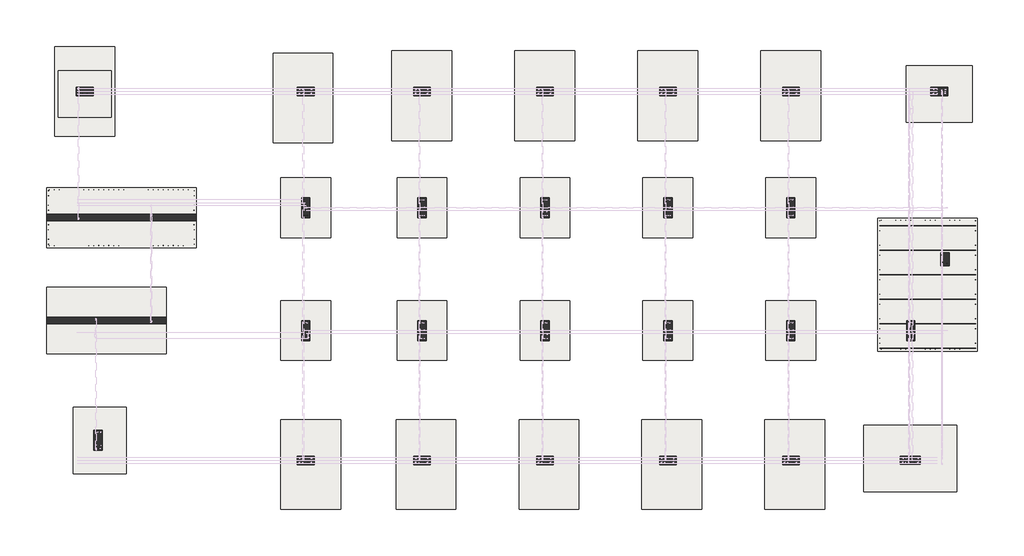
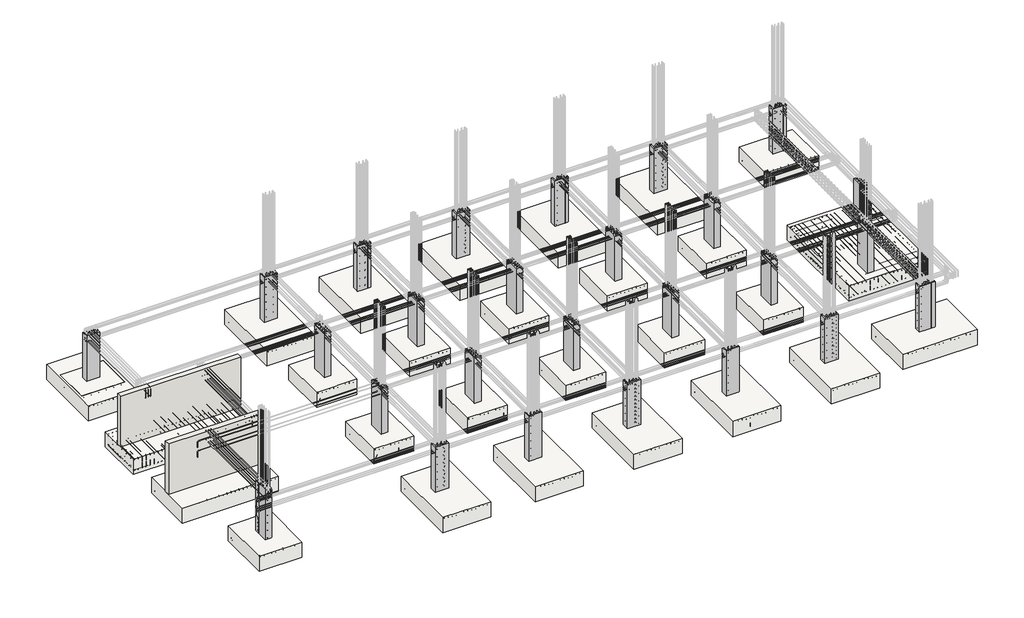
# One storey, part 1 of 18: 28 slabs, 27 columns, 3 walls.
"""IFC4 building model written with IfcOpenShell, lengths in millimetres."""

from ifc_helpers import new_model, si_unit, frame, origin, place, context, project, spatial, polyline, outline, extrude, faceted_brep, transform, mapped, element, save
from components import m_footing_rectangular_1500x1800x600_40ea0b3e, m_footing_rectangular_1800x2700x600_14f11077, m_footing_rectangular_1800x4498x600_2b6d0f7f, m_footing_rectangular_2000x1600x600_a227f129, m_footing_rectangular_2000x1700x600_e7f9a9ee, m_footing_rectangular_2000x3600x600_ead935d4, m_footing_rectangular_2800x2000x600_85f03661, m_footing_rectangular_3000x4000x600_f1bd0d4a

model = new_model("IFC4")

# Units and contexts
model_context = context("Model", 3, world=origin())
ifc_project = project(units=[si_unit("LENGTHUNIT", "METRE", prefix="MILLI")], contexts=[model_context])

# Site, building, storey
site = spatial("IfcSite", under=ifc_project)
building = spatial("IfcBuilding", under=site)
storey = spatial("IfcBuildingStorey", under=building, Elevation=-2000.0)

# Columns
placement = place(None, origin())
element("IfcColumn", 1, ObjectType="M_Concrete-Rectangular-Column : 400X250", at=placement, inside=storey, context=model_context, shape_type="Brep", body=[
    faceted_brep([(10445.870951, 692.5978854, -2000.0), (10695.870951, 692.5978854, -2000.0), (10695.870951, 292.5978854, -2000.0), (10445.870951, 292.5978854, -2000.0), (10445.870951, 692.5978854, -500.0), (10445.870951, 692.5978854, -210.0), (10695.870951, 692.5978854, -210.0), (10695.870951, 692.5978854, -500.0), (10695.870951, 292.5978854, -210.0), (10695.870951, 292.5978854, -500.0), (10445.870951, 292.5978854, -210.0), (10445.870951, 292.5978854, -500.0)], [[[0, 1, 2, 3]], [[1, 0, 4, 5, 6, 7]], [[2, 1, 7, 6, 8, 9]], [[3, 2, 9, 8, 10, 11]], [[0, 3, 11, 10, 5, 4]], [[6, 5, 10, 8]]]),
])
element("IfcColumn", 2, ObjectType="M_Concrete-Rectangular-Column : 500X250", at=placement, inside=storey, context=model_context, shape_type="SweptSolid", body=[
    extrude(outline(polyline([(-15070.6290491, 5667.5978854), (-15070.6290491, 5417.5978854), (-15570.6290491, 5417.5978854), (-15570.6290491, 5667.5978854), (-15070.6290491, 5667.5978854)])), frame((0.0, 0.0, -2000.0), z_axis=(0.0, 0.0, 1.0), x_axis=(1.0, 0.0, 0.0)), (0.0, 0.0, 1.0), 1790.0),
])
element("IfcColumn", 3, ObjectType="M_Concrete-Rectangular-Column : 500X250", at=placement, inside=storey, context=model_context, shape_type="Brep", body=[
    faceted_brep([(-15070.6290491, 5667.5978854, -2000.0), (-15070.6290491, 5417.5978854, -2000.0), (-15570.6290491, 5417.5978854, -2000.0), (-15570.6290491, 5667.5978854, -2000.0), (-15070.6290491, 5667.5978854, -500.0), (-15070.6290491, 5667.5978854, -210.0), (-15070.6290491, 5417.5978854, -210.0), (-15070.6290491, 5417.5978854, -500.0), (-15570.6290491, 5417.5978854, -210.0), (-15570.6290491, 5417.5978854, -500.0), (-15570.6290491, 5667.5978854, -210.0), (-15570.6290491, 5667.5978854, -500.0)], [[[0, 1, 2, 3]], [[1, 0, 4, 5, 6, 7]], [[2, 1, 7, 6, 8, 9]], [[3, 2, 9, 8, 10, 11]], [[0, 3, 11, 10, 5, 4]], [[6, 5, 10, 8]]]),
])
element("IfcColumn", 4, ObjectType="M_Concrete-Rectangular-Column : 500X250", at=placement, inside=storey, context=model_context, shape_type="Brep", body=[
    faceted_brep([(-8420.5899692, 5667.5978854, -2000.0), (-8420.5899692, 5417.5978854, -2000.0), (-8920.5899692, 5417.5978854, -2000.0), (-8920.5899692, 5667.5978854, -2000.0), (-8420.5899692, 5667.5978854, -500.0), (-8420.5899692, 5667.5978854, -210.0), (-8420.5899692, 5417.5978854, -210.0), (-8420.5899692, 5417.5978854, -500.0), (-8920.5899692, 5417.5978854, -210.0), (-8920.5899692, 5417.5978854, -500.0), (-8920.5899692, 5667.5978854, -210.0), (-8920.5899692, 5667.5978854, -500.0)], [[[0, 1, 2, 3]], [[1, 0, 4, 5, 6, 7]], [[2, 1, 7, 6, 8, 9]], [[3, 2, 9, 8, 10, 11]], [[0, 3, 11, 10, 5, 4]], [[6, 5, 10, 8]]]),
])
element("IfcColumn", 5, ObjectType="M_Concrete-Rectangular-Column : 500X250", at=placement, inside=storey, context=model_context, shape_type="Brep", body=[
    faceted_brep([(-4920.5899692, 5667.5978854, -2000.0), (-4920.5899692, 5417.5978854, -2000.0), (-5420.5899692, 5417.5978854, -2000.0), (-5420.5899692, 5667.5978854, -2000.0), (-4920.5899692, 5667.5978854, -500.0), (-4920.5899692, 5667.5978854, -210.0), (-4920.5899692, 5417.5978854, -210.0), (-4920.5899692, 5417.5978854, -500.0), (-5420.5899692, 5417.5978854, -210.0), (-5420.5899692, 5417.5978854, -500.0), (-5420.5899692, 5667.5978854, -210.0), (-5420.5899692, 5667.5978854, -500.0)], [[[0, 1, 2, 3]], [[1, 0, 4, 5, 6, 7]], [[2, 1, 7, 6, 8, 9]], [[3, 2, 9, 8, 10, 11]], [[0, 3, 11, 10, 5, 4]], [[6, 5, 10, 8]]]),
])
element("IfcColumn", 6, ObjectType="M_Concrete-Rectangular-Column : 500X250", at=placement, inside=storey, context=model_context, shape_type="Brep", body=[
    faceted_brep([(-1220.5899692, 5667.5978854, -2000.0), (-1220.5899692, 5417.5978854, -2000.0), (-1720.5899692, 5417.5978854, -2000.0), (-1720.5899692, 5667.5978854, -2000.0), (-1220.5899692, 5667.5978854, -500.0), (-1220.5899692, 5667.5978854, -210.0), (-1220.5899692, 5417.5978854, -210.0), (-1220.5899692, 5417.5978854, -500.0), (-1720.5899692, 5417.5978854, -210.0), (-1720.5899692, 5417.5978854, -500.0), (-1720.5899692, 5667.5978854, -210.0), (-1720.5899692, 5667.5978854, -500.0)], [[[0, 1, 2, 3]], [[1, 0, 4, 5, 6, 7]], [[2, 1, 7, 6, 8, 9]], [[3, 2, 9, 8, 10, 11]], [[0, 3, 11, 10, 5, 4]], [[6, 5, 10, 8]]]),
])
element("IfcColumn", 7, ObjectType="M_Concrete-Rectangular-Column : 500X250", at=placement, inside=storey, context=model_context, shape_type="Brep", body=[
    faceted_brep([(2479.4100308, 5667.5978854, -2000.0), (2479.4100308, 5417.5978854, -2000.0), (1979.4100308, 5417.5978854, -2000.0), (1979.4100308, 5667.5978854, -2000.0), (2479.4100308, 5667.5978854, -500.0), (2479.4100308, 5667.5978854, -210.0), (2479.4100308, 5417.5978854, -210.0), (2479.4100308, 5417.5978854, -500.0), (1979.4100308, 5417.5978854, -210.0), (1979.4100308, 5417.5978854, -500.0), (1979.4100308, 5667.5978854, -210.0), (1979.4100308, 5667.5978854, -500.0)], [[[0, 1, 2, 3]], [[1, 0, 4, 5, 6, 7]], [[2, 1, 7, 6, 8, 9]], [[3, 2, 9, 8, 10, 11]], [[0, 3, 11, 10, 5, 4]], [[6, 5, 10, 8]]]),
])
element("IfcColumn", 8, ObjectType="M_Concrete-Rectangular-Column : 500X250", at=placement, inside=storey, context=model_context, shape_type="Brep", body=[
    faceted_brep([(6179.4100308, 5667.5978854, -2000.0), (6179.4100308, 5417.5978854, -2000.0), (5679.4100308, 5417.5978854, -2000.0), (5679.4100308, 5667.5978854, -2000.0), (6179.4100308, 5667.5978854, -500.0), (6179.4100308, 5667.5978854, -210.0), (6179.4100308, 5417.5978854, -210.0), (6179.4100308, 5417.5978854, -500.0), (5679.4100308, 5417.5978854, -210.0), (5679.4100308, 5417.5978854, -500.0), (5679.4100308, 5667.5978854, -210.0), (5679.4100308, 5667.5978854, -500.0)], [[[0, 1, 2, 3]], [[1, 0, 4, 5, 6, 7]], [[2, 1, 7, 6, 8, 9]], [[3, 2, 9, 8, 10, 11]], [[0, 3, 11, 10, 5, 4]], [[6, 5, 10, 8]]]),
])
element("IfcColumn", 9, ObjectType="M_Concrete-Rectangular-Column : 500X250", at=placement, inside=storey, context=model_context, shape_type="SweptSolid", body=[
    extrude(outline(polyline([(10645.870951, 5667.5978854), (10645.870951, 5417.5978854), (10145.870951, 5417.5978854), (10145.870951, 5667.5978854), (10645.870951, 5667.5978854)])), frame((0.0, 0.0, -2000.0), z_axis=(0.0, 0.0, 1.0), x_axis=(1.0, 0.0, 0.0)), (0.0, 0.0, 1.0), 1790.0),
])
element("IfcColumn", 10, ObjectType="M_Concrete-Rectangular-Column : 500X250", at=placement, inside=storey, context=model_context, shape_type="Brep", body=[
    faceted_brep([(-8420.5899692, -5436.6797656, -2000.0), (-8420.5899692, -5686.6797656, -2000.0), (-8920.5899692, -5686.6797656, -2000.0), (-8920.5899692, -5436.6797656, -2000.0), (-8420.5899692, -5436.6797656, -500.0), (-8420.5899692, -5436.6797656, -210.0), (-8420.5899692, -5686.6797656, -210.0), (-8420.5899692, -5686.6797656, -500.0), (-8920.5899692, -5686.6797656, -210.0), (-8920.5899692, -5686.6797656, -500.0), (-8920.5899692, -5436.6797656, -210.0), (-8920.5899692, -5436.6797656, -500.0)], [[[0, 1, 2, 3]], [[1, 0, 4, 5, 6, 7]], [[2, 1, 7, 6, 8, 9]], [[3, 2, 9, 8, 10, 11]], [[0, 3, 11, 10, 5, 4]], [[6, 5, 10, 8]]]),
])
element("IfcColumn", 11, ObjectType="M_Concrete-Rectangular-Column : 500X250", at=placement, inside=storey, context=model_context, shape_type="Brep", body=[
    faceted_brep([(-4920.5899692, -5436.6797656, -2000.0), (-4920.5899692, -5686.6797656, -2000.0), (-5420.5899692, -5686.6797656, -2000.0), (-5420.5899692, -5436.6797656, -2000.0), (-4920.5899692, -5436.6797656, -500.0), (-4920.5899692, -5436.6797656, -210.0), (-4920.5899692, -5686.6797656, -210.0), (-4920.5899692, -5686.6797656, -500.0), (-5420.5899692, -5686.6797656, -210.0), (-5420.5899692, -5686.6797656, -500.0), (-5420.5899692, -5436.6797656, -210.0), (-5420.5899692, -5436.6797656, -500.0)], [[[0, 1, 2, 3]], [[1, 0, 4, 5, 6, 7]], [[2, 1, 7, 6, 8, 9]], [[3, 2, 9, 8, 10, 11]], [[0, 3, 11, 10, 5, 4]], [[6, 5, 10, 8]]]),
])
element("IfcColumn", 12, ObjectType="M_Concrete-Rectangular-Column : 500X250", at=placement, inside=storey, context=model_context, shape_type="Brep", body=[
    faceted_brep([(-1220.5899692, -5436.6797656, -2000.0), (-1220.5899692, -5686.6797656, -2000.0), (-1720.5899692, -5686.6797656, -2000.0), (-1720.5899692, -5436.6797656, -2000.0), (-1220.5899692, -5436.6797656, -500.0), (-1220.5899692, -5436.6797656, -210.0), (-1220.5899692, -5686.6797656, -210.0), (-1220.5899692, -5686.6797656, -500.0), (-1720.5899692, -5686.6797656, -210.0), (-1720.5899692, -5686.6797656, -500.0), (-1720.5899692, -5436.6797656, -210.0), (-1720.5899692, -5436.6797656, -500.0)], [[[0, 1, 2, 3]], [[1, 0, 4, 5, 6, 7]], [[2, 1, 7, 6, 8, 9]], [[3, 2, 9, 8, 10, 11]], [[0, 3, 11, 10, 5, 4]], [[6, 5, 10, 8]]]),
])
element("IfcColumn", 13, ObjectType="M_Concrete-Rectangular-Column : 500X250", at=placement, inside=storey, context=model_context, shape_type="Brep", body=[
    faceted_brep([(2479.4100308, -5436.6797656, -2000.0), (2479.4100308, -5686.6797656, -2000.0), (1979.4100308, -5686.6797656, -2000.0), (1979.4100308, -5436.6797656, -2000.0), (2479.4100308, -5436.6797656, -500.0), (2479.4100308, -5436.6797656, -210.0), (2479.4100308, -5686.6797656, -210.0), (2479.4100308, -5686.6797656, -500.0), (1979.4100308, -5686.6797656, -210.0), (1979.4100308, -5686.6797656, -500.0), (1979.4100308, -5436.6797656, -210.0), (1979.4100308, -5436.6797656, -500.0)], [[[0, 1, 2, 3]], [[1, 0, 4, 5, 6, 7]], [[2, 1, 7, 6, 8, 9]], [[3, 2, 9, 8, 10, 11]], [[0, 3, 11, 10, 5, 4]], [[6, 5, 10, 8]]]),
])
element("IfcColumn", 14, ObjectType="M_Concrete-Rectangular-Column : 500X250", at=placement, inside=storey, context=model_context, shape_type="Brep", body=[
    faceted_brep([(6179.4100308, -5436.6797656, -2000.0), (6179.4100308, -5686.6797656, -2000.0), (5679.4100308, -5686.6797656, -2000.0), (5679.4100308, -5436.6797656, -2000.0), (6179.4100308, -5436.6797656, -500.0), (6179.4100308, -5436.6797656, -210.0), (6179.4100308, -5686.6797656, -210.0), (6179.4100308, -5686.6797656, -500.0), (5679.4100308, -5686.6797656, -210.0), (5679.4100308, -5686.6797656, -500.0), (5679.4100308, -5436.6797656, -210.0), (5679.4100308, -5436.6797656, -500.0)], [[[0, 1, 2, 3]], [[1, 0, 4, 5, 6, 7]], [[2, 1, 7, 6, 8, 9]], [[3, 2, 9, 8, 10, 11]], [[0, 3, 11, 10, 5, 4]], [[6, 5, 10, 8]]]),
])
element("IfcColumn", 15, ObjectType="M_Concrete-Rectangular-Column : 600X250", at=placement, inside=storey, context=model_context, shape_type="Brep", body=[
    faceted_brep([(9825.870951, -5431.4021146, -2000.0), (9825.870951, -5681.4021146, -2000.0), (9225.870951, -5681.4021146, -2000.0), (9225.870951, -5431.4021146, -2000.0), (9825.870951, -5431.4021146, -500.0), (9825.870951, -5431.4021146, -210.0), (9825.870951, -5681.4021146, -210.0), (9825.870951, -5681.4021146, -500.0), (9225.870951, -5681.4021146, -210.0), (9225.870951, -5681.4021146, -500.0), (9225.870951, -5431.4021146, -210.0), (9225.870951, -5431.4021146, -500.0)], [[[0, 1, 2, 3]], [[1, 0, 4, 5, 6, 7]], [[2, 1, 7, 6, 8, 9]], [[3, 2, 9, 8, 10, 11]], [[0, 3, 11, 10, 5, 4]], [[6, 5, 10, 8]]]),
])
element("IfcColumn", 16, ObjectType="M_Concrete-Rectangular-Column : 600X250", at=placement, inside=storey, context=model_context, shape_type="Brep", body=[
    faceted_brep([(9414.6559943, -1357.4021146, -2000.0), (9664.6559943, -1357.4021146, -2000.0), (9664.6559943, -1957.4021146, -2000.0), (9414.6559943, -1957.4021146, -2000.0), (9414.6559943, -1357.4021146, -210.0), (9439.6559943, -1357.4021146, -210.0), (9639.6559943, -1357.4021146, -210.0), (9664.6559943, -1357.4021146, -210.0), (9664.6559943, -1507.4021146, -210.0), (9664.6559943, -1807.4021146, -210.0), (9664.6559943, -1957.4021146, -210.0), (9639.6559943, -1957.4021146, -210.0), (9439.6559943, -1957.4021146, -210.0), (9414.6559943, -1957.4021146, -210.0), (9414.6559943, -1807.4021146, -210.0), (9414.6559943, -1507.4021146, -210.0)], [[[0, 1, 2, 3]], [[1, 0, 4, 5, 6, 7]], [[2, 1, 7, 8, 9, 10]], [[3, 2, 10, 11, 12, 13]], [[0, 3, 13, 14, 15, 4]], [[7, 6, 5, 4, 15, 14, 13, 12, 11, 10, 9, 8]]]),
])
element("IfcColumn", 17, ObjectType="M_Concrete-Rectangular-Column : 600X250", at=placement, inside=storey, context=model_context, shape_type="Brep", body=[
    faceted_brep([(5804.4100308, -1357.4021146, -2000.0), (6054.4100308, -1357.4021146, -2000.0), (6054.4100308, -1957.4021146, -2000.0), (5804.4100308, -1957.4021146, -2000.0), (5804.4100308, -1357.4021146, -500.0), (5804.4100308, -1357.4021146, -210.0), (6054.4100308, -1357.4021146, -210.0), (6054.4100308, -1357.4021146, -500.0), (6054.4100308, -1507.4021146, -210.0), (6054.4100308, -1807.4021146, -210.0), (6054.4100308, -1957.4021146, -210.0), (6054.4100308, -1957.4021146, -500.0), (5804.4100308, -1957.4021146, -210.0), (5804.4100308, -1957.4021146, -500.0), (5804.4100308, -1807.4021146, -210.0), (5804.4100308, -1507.4021146, -210.0)], [[[0, 1, 2, 3]], [[1, 0, 4, 5, 6, 7]], [[2, 1, 7, 6, 8, 9, 10, 11]], [[3, 2, 11, 10, 12, 13]], [[0, 3, 13, 12, 14, 15, 5, 4]], [[6, 5, 15, 14, 12, 10, 9, 8]]]),
])
element("IfcColumn", 18, ObjectType="M_Concrete-Rectangular-Column : 600X250", at=placement, inside=storey, context=model_context, shape_type="Brep", body=[
    faceted_brep([(2104.4100308, -1357.4021146, -2000.0), (2354.4100308, -1357.4021146, -2000.0), (2354.4100308, -1957.4021146, -2000.0), (2104.4100308, -1957.4021146, -2000.0), (2104.4100308, -1357.4021146, -500.0), (2104.4100308, -1357.4021146, -210.0), (2354.4100308, -1357.4021146, -210.0), (2354.4100308, -1357.4021146, -500.0), (2354.4100308, -1507.4021146, -210.0), (2354.4100308, -1807.4021146, -210.0), (2354.4100308, -1957.4021146, -210.0), (2354.4100308, -1957.4021146, -500.0), (2104.4100308, -1957.4021146, -210.0), (2104.4100308, -1957.4021146, -500.0), (2104.4100308, -1807.4021146, -210.0), (2104.4100308, -1507.4021146, -210.0)], [[[0, 1, 2, 3]], [[1, 0, 4, 5, 6, 7]], [[2, 1, 7, 6, 8, 9, 10, 11]], [[3, 2, 11, 10, 12, 13]], [[0, 3, 13, 12, 14, 15, 5, 4]], [[6, 5, 15, 14, 12, 10, 9, 8]]]),
])
element("IfcColumn", 19, ObjectType="M_Concrete-Rectangular-Column : 600X250", at=placement, inside=storey, context=model_context, shape_type="Brep", body=[
    faceted_brep([(-5295.5899692, -1357.4021146, -2000.0), (-5045.5899692, -1357.4021146, -2000.0), (-5045.5899692, -1957.4021146, -2000.0), (-5295.5899692, -1957.4021146, -2000.0), (-5295.5899692, -1357.4021146, -500.0), (-5295.5899692, -1357.4021146, -210.0), (-5045.5899692, -1357.4021146, -210.0), (-5045.5899692, -1357.4021146, -500.0), (-5045.5899692, -1507.4021146, -210.0), (-5045.5899692, -1807.4021146, -210.0), (-5045.5899692, -1957.4021146, -210.0), (-5045.5899692, -1957.4021146, -500.0), (-5295.5899692, -1957.4021146, -210.0), (-5295.5899692, -1957.4021146, -500.0), (-5295.5899692, -1807.4021146, -210.0), (-5295.5899692, -1507.4021146, -210.0)], [[[0, 1, 2, 3]], [[1, 0, 4, 5, 6, 7]], [[2, 1, 7, 6, 8, 9, 10, 11]], [[3, 2, 11, 10, 12, 13]], [[0, 3, 13, 12, 14, 15, 5, 4]], [[6, 5, 15, 14, 12, 10, 9, 8]]]),
])
element("IfcColumn", 20, ObjectType="M_Concrete-Rectangular-Column : 600X250", at=placement, inside=storey, context=model_context, shape_type="Brep", body=[
    faceted_brep([(-1595.5899692, -1357.4021146, -2000.0), (-1345.5899692, -1357.4021146, -2000.0), (-1345.5899692, -1957.4021146, -2000.0), (-1595.5899692, -1957.4021146, -2000.0), (-1595.5899692, -1357.4021146, -500.0), (-1595.5899692, -1357.4021146, -210.0), (-1345.5899692, -1357.4021146, -210.0), (-1345.5899692, -1357.4021146, -500.0), (-1345.5899692, -1507.4021146, -210.0), (-1345.5899692, -1807.4021146, -210.0), (-1345.5899692, -1957.4021146, -210.0), (-1345.5899692, -1957.4021146, -500.0), (-1595.5899692, -1957.4021146, -210.0), (-1595.5899692, -1957.4021146, -500.0), (-1595.5899692, -1807.4021146, -210.0), (-1595.5899692, -1507.4021146, -210.0)], [[[0, 1, 2, 3]], [[1, 0, 4, 5, 6, 7]], [[2, 1, 7, 6, 8, 9, 10, 11]], [[3, 2, 11, 10, 12, 13]], [[0, 3, 13, 12, 14, 15, 5, 4]], [[6, 5, 15, 14, 12, 10, 9, 8]]]),
])
element("IfcColumn", 21, ObjectType="M_Concrete-Rectangular-Column : 600X250", at=placement, inside=storey, context=model_context, shape_type="Brep", body=[
    faceted_brep([(-8795.5899692, -1357.4021146, -2000.0), (-8545.5899692, -1357.4021146, -2000.0), (-8545.5899692, -1957.4021146, -2000.0), (-8795.5899692, -1957.4021146, -2000.0), (-8795.5899692, -1357.4021146, -500.0), (-8795.5899692, -1357.4021146, -210.0), (-8545.5899692, -1357.4021146, -210.0), (-8545.5899692, -1357.4021146, -500.0), (-8545.5899692, -1957.4021146, -210.0), (-8545.5899692, -1957.4021146, -500.0), (-8795.5899692, -1957.4021146, -210.0), (-8795.5899692, -1957.4021146, -500.0)], [[[0, 1, 2, 3]], [[1, 0, 4, 5, 6, 7]], [[2, 1, 7, 6, 8, 9]], [[3, 2, 9, 8, 10, 11]], [[0, 3, 11, 10, 5, 4]], [[6, 5, 10, 8]]]),
])
element("IfcColumn", 22, ObjectType="M_Concrete-Rectangular-Column : 600X250", at=placement, inside=storey, context=model_context, shape_type="Brep", body=[
    faceted_brep([(-8795.5899692, 2342.5978854, -2000.0), (-8545.5899692, 2342.5978854, -2000.0), (-8545.5899692, 1742.5978854, -2000.0), (-8795.5899692, 1742.5978854, -2000.0), (-8795.5899692, 2342.5978854, -500.0), (-8795.5899692, 2342.5978854, -210.0), (-8545.5899692, 2342.5978854, -210.0), (-8545.5899692, 2342.5978854, -500.0), (-8545.5899692, 1742.5978854, -210.0), (-8545.5899692, 1742.5978854, -500.0), (-8795.5899692, 1742.5978854, -210.0), (-8795.5899692, 1742.5978854, -500.0)], [[[0, 1, 2, 3]], [[1, 0, 4, 5, 6, 7]], [[2, 1, 7, 6, 8, 9]], [[3, 2, 9, 8, 10, 11]], [[0, 3, 11, 10, 5, 4]], [[6, 5, 10, 8]]]),
])
element("IfcColumn", 23, ObjectType="M_Concrete-Rectangular-Column : 600X250", at=placement, inside=storey, context=model_context, shape_type="Brep", body=[
    faceted_brep([(-5295.5899692, 2342.5978854, -2000.0), (-5045.5899692, 2342.5978854, -2000.0), (-5045.5899692, 1742.5978854, -2000.0), (-5295.5899692, 1742.5978854, -2000.0), (-5295.5899692, 2342.5978854, -500.0), (-5295.5899692, 2342.5978854, -210.0), (-5045.5899692, 2342.5978854, -210.0), (-5045.5899692, 2342.5978854, -500.0), (-5045.5899692, 2192.5978854, -210.0), (-5045.5899692, 1892.5978854, -210.0), (-5045.5899692, 1742.5978854, -210.0), (-5045.5899692, 1742.5978854, -500.0), (-5295.5899692, 1742.5978854, -210.0), (-5295.5899692, 1742.5978854, -500.0), (-5295.5899692, 1892.5978854, -210.0), (-5295.5899692, 2192.5978854, -210.0)], [[[0, 1, 2, 3]], [[1, 0, 4, 5, 6, 7]], [[2, 1, 7, 6, 8, 9, 10, 11]], [[3, 2, 11, 10, 12, 13]], [[0, 3, 13, 12, 14, 15, 5, 4]], [[6, 5, 15, 14, 12, 10, 9, 8]]]),
])
element("IfcColumn", 24, ObjectType="M_Concrete-Rectangular-Column : 600X250", at=placement, inside=storey, context=model_context, shape_type="Brep", body=[
    faceted_brep([(-1595.5899692, 2342.5978854, -2000.0), (-1345.5899692, 2342.5978854, -2000.0), (-1345.5899692, 1742.5978854, -2000.0), (-1595.5899692, 1742.5978854, -2000.0), (-1595.5899692, 2342.5978854, -500.0), (-1595.5899692, 2342.5978854, -210.0), (-1345.5899692, 2342.5978854, -210.0), (-1345.5899692, 2342.5978854, -500.0), (-1345.5899692, 2192.5978854, -210.0), (-1345.5899692, 1892.5978854, -210.0), (-1345.5899692, 1742.5978854, -210.0), (-1345.5899692, 1742.5978854, -500.0), (-1595.5899692, 1742.5978854, -210.0), (-1595.5899692, 1742.5978854, -500.0), (-1595.5899692, 1892.5978854, -210.0), (-1595.5899692, 2192.5978854, -210.0)], [[[0, 1, 2, 3]], [[1, 0, 4, 5, 6, 7]], [[2, 1, 7, 6, 8, 9, 10, 11]], [[3, 2, 11, 10, 12, 13]], [[0, 3, 13, 12, 14, 15, 5, 4]], [[6, 5, 15, 14, 12, 10, 9, 8]]]),
])
element("IfcColumn", 25, ObjectType="M_Concrete-Rectangular-Column : 600X250", at=placement, inside=storey, context=model_context, shape_type="Brep", body=[
    faceted_brep([(2104.4100308, 2342.5978854, -2000.0), (2354.4100308, 2342.5978854, -2000.0), (2354.4100308, 1742.5978854, -2000.0), (2104.4100308, 1742.5978854, -2000.0), (2104.4100308, 2342.5978854, -500.0), (2104.4100308, 2342.5978854, -210.0), (2354.4100308, 2342.5978854, -210.0), (2354.4100308, 2342.5978854, -500.0), (2354.4100308, 2192.5978854, -210.0), (2354.4100308, 1892.5978854, -210.0), (2354.4100308, 1742.5978854, -210.0), (2354.4100308, 1742.5978854, -500.0), (2104.4100308, 1742.5978854, -210.0), (2104.4100308, 1742.5978854, -500.0), (2104.4100308, 1892.5978854, -210.0), (2104.4100308, 2192.5978854, -210.0)], [[[0, 1, 2, 3]], [[1, 0, 4, 5, 6, 7]], [[2, 1, 7, 6, 8, 9, 10, 11]], [[3, 2, 11, 10, 12, 13]], [[0, 3, 13, 12, 14, 15, 5, 4]], [[6, 5, 15, 14, 12, 10, 9, 8]]]),
])
element("IfcColumn", 26, ObjectType="M_Concrete-Rectangular-Column : 600X250", at=placement, inside=storey, context=model_context, shape_type="Brep", body=[
    faceted_brep([(5804.4100308, 2342.5978854, -2000.0), (6054.4100308, 2342.5978854, -2000.0), (6054.4100308, 1742.5978854, -2000.0), (5804.4100308, 1742.5978854, -2000.0), (5804.4100308, 2342.5978854, -500.0), (5804.4100308, 2342.5978854, -210.0), (6054.4100308, 2342.5978854, -210.0), (6054.4100308, 2342.5978854, -500.0), (6054.4100308, 2192.5978854, -210.0), (6054.4100308, 1892.5978854, -210.0), (6054.4100308, 1742.5978854, -210.0), (6054.4100308, 1742.5978854, -500.0), (5804.4100308, 1742.5978854, -210.0), (5804.4100308, 1742.5978854, -500.0), (5804.4100308, 1892.5978854, -210.0), (5804.4100308, 2192.5978854, -210.0)], [[[0, 1, 2, 3]], [[1, 0, 4, 5, 6, 7]], [[2, 1, 7, 6, 8, 9, 10, 11]], [[3, 2, 11, 10, 12, 13]], [[0, 3, 13, 12, 14, 15, 5, 4]], [[6, 5, 15, 14, 12, 10, 9, 8]]]),
])
element("IfcColumn", 27, ObjectType="M_Concrete-Rectangular-Column : 600X250", at=placement, inside=storey, context=model_context, shape_type="Brep", body=[
    faceted_brep([(-15042.8702104, -4657.4021146, -2000.0), (-14792.8702104, -4657.4021146, -2000.0), (-14792.8702104, -5257.4021146, -2000.0), (-15042.8702104, -5257.4021146, -2000.0), (-15042.8702104, -4657.4021146, -500.0), (-15042.8702104, -4657.4021146, 0.0), (-15039.129049, -4657.4021146, 0.0), (-15039.129049, -4657.4021146, -210.0), (-14792.8702104, -4657.4021146, -210.0), (-14792.8702104, -4657.4021146, -500.0), (-14792.8702104, -5257.4021146, -210.0), (-14792.8702104, -5257.4021146, -500.0), (-15039.129049, -5257.4021146, -210.0), (-15039.129049, -5257.4021146, 0.0), (-15042.8702104, -5257.4021146, 0.0), (-15042.8702104, -5257.4021146, -500.0)], [[[0, 1, 2, 3]], [[1, 0, 4, 5, 6, 7, 8, 9]], [[2, 1, 9, 8, 10, 11]], [[3, 2, 11, 10, 12, 13, 14, 15]], [[0, 3, 15, 14, 5, 4]], [[5, 14, 13, 6]], [[7, 12, 10, 8]], [[12, 7, 6, 13]]]),
])

# Slabs
m_footing_rectangular_1500x1800x600_shape = m_footing_rectangular_1500x1800x600_40ea0b3e(model_context)
element("IfcSlab", 28, ObjectType="M_Footing-Rectangular : 1500X1800X600", at=placement, inside=storey, context=model_context, shape_type="MappedRepresentation", body=[
    mapped(m_footing_rectangular_1500x1800x600_shape, transform((-8671.6414888, 2044.0399624, -2000.0), x_axis=(1.0, 0.0, 0.0), y_axis=(0.0, 1.0, 0.0), z_axis=(0.0, 0.0, 1.0))),
])
element("IfcSlab", 29, ObjectType="M_Footing-Rectangular : 1500X1800X600", at=placement, inside=storey, context=model_context, shape_type="MappedRepresentation", body=[
    mapped(m_footing_rectangular_1500x1800x600_shape, transform((-5170.5899692, 2045.4820394, -2000.0), x_axis=(1.0, 0.0, 0.0), y_axis=(0.0, 1.0, 0.0), z_axis=(0.0, 0.0, 1.0))),
])
element("IfcSlab", 30, ObjectType="M_Footing-Rectangular : 1500X1800X600", at=placement, inside=storey, context=model_context, shape_type="MappedRepresentation", body=[
    mapped(m_footing_rectangular_1500x1800x600_shape, transform((-1470.5899692, 2045.4820394, -2000.0), x_axis=(1.0, 0.0, 0.0), y_axis=(0.0, 1.0, 0.0), z_axis=(0.0, 0.0, 1.0))),
])
element("IfcSlab", 31, ObjectType="M_Footing-Rectangular : 1500X1800X600", at=placement, inside=storey, context=model_context, shape_type="MappedRepresentation", body=[
    mapped(m_footing_rectangular_1500x1800x600_shape, transform((2229.4100308, 2045.4820394, -2000.0), x_axis=(1.0, 0.0, 0.0), y_axis=(0.0, 1.0, 0.0), z_axis=(0.0, 0.0, 1.0))),
])
element("IfcSlab", 32, ObjectType="M_Footing-Rectangular : 1500X1800X600", at=placement, inside=storey, context=model_context, shape_type="MappedRepresentation", body=[
    mapped(m_footing_rectangular_1500x1800x600_shape, transform((5929.4100308, 2045.4820394, -2000.0), x_axis=(1.0, 0.0, 0.0), y_axis=(0.0, 1.0, 0.0), z_axis=(0.0, 0.0, 1.0))),
])
element("IfcSlab", 33, ObjectType="M_Footing-Rectangular : 1500X1800X600", at=placement, inside=storey, context=model_context, shape_type="MappedRepresentation", body=[
    mapped(m_footing_rectangular_1500x1800x600_shape, transform((5929.4100308, -1655.9600376, -2000.0), x_axis=(1.0, 0.0, 0.0), y_axis=(0.0, 1.0, 0.0), z_axis=(0.0, 0.0, 1.0))),
])
element("IfcSlab", 34, ObjectType="M_Footing-Rectangular : 1500X1800X600", at=placement, inside=storey, context=model_context, shape_type="MappedRepresentation", body=[
    mapped(m_footing_rectangular_1500x1800x600_shape, transform((2229.4100308, -1655.9600376, -2000.0), x_axis=(1.0, 0.0, 0.0), y_axis=(0.0, 1.0, 0.0), z_axis=(0.0, 0.0, 1.0))),
])
element("IfcSlab", 35, ObjectType="M_Footing-Rectangular : 1500X1800X600", at=placement, inside=storey, context=model_context, shape_type="MappedRepresentation", body=[
    mapped(m_footing_rectangular_1500x1800x600_shape, transform((-1470.5899692, -1655.9600376, -2000.0), x_axis=(1.0, 0.0, 0.0), y_axis=(0.0, 1.0, 0.0), z_axis=(0.0, 0.0, 1.0))),
])
element("IfcSlab", 36, ObjectType="M_Footing-Rectangular : 1500X1800X600", at=placement, inside=storey, context=model_context, shape_type="MappedRepresentation", body=[
    mapped(m_footing_rectangular_1500x1800x600_shape, transform((-5170.5899692, -1655.9600376, -2000.0), x_axis=(1.0, 0.0, 0.0), y_axis=(0.0, 1.0, 0.0), z_axis=(0.0, 0.0, 1.0))),
])
element("IfcSlab", 37, ObjectType="M_Footing-Rectangular : 1500X1800X600", at=placement, inside=storey, context=model_context, shape_type="MappedRepresentation", body=[
    mapped(m_footing_rectangular_1500x1800x600_shape, transform((-8670.5899692, -1655.9600376, -2000.0), x_axis=(1.0, 0.0, 0.0), y_axis=(0.0, 1.0, 0.0), z_axis=(0.0, 0.0, 1.0))),
])
element("IfcSlab", 38, ObjectType="M_Footing-Rectangular : 1600X1400X600", at=placement, inside=storey, context=model_context, shape_type="SweptSolid", body=[
    extrude(outline(polyline([(-14520.6290491, 6167.5978854), (-14520.6290491, 4767.5978854), (-16120.6290491, 4767.5978854), (-16120.6290491, 6167.5978854), (-14520.6290491, 6167.5978854)])), frame((0.0, 0.0, -2600.0), z_axis=(0.0, 0.0, 1.0), x_axis=(1.0, 0.0, 0.0)), (0.0, 0.0, 1.0), 600.0),
])
element("IfcSlab", 39, ObjectType="M_Footing-Rectangular : 1800X2700X600", at=placement, inside=storey, context=model_context, shape_type="SweptSolid", body=[
    extrude(outline(polyline([(-14420.6290491, 6892.5978854), (-14420.6290491, 4192.5978854), (-16220.6290491, 4192.5978854), (-16220.6290491, 6892.5978854), (-14420.6290491, 6892.5978854)]), holes=[polyline([(-14520.6290491, 6167.5978854), (-16120.6290491, 6167.5978854), (-16120.6290491, 4767.5978854), (-14520.6290491, 4767.5978854), (-14520.6290491, 6167.5978854)])]), frame((0.0, 0.0, -2600.0), z_axis=(0.0, 0.0, 1.0), x_axis=(1.0, 0.0, 0.0)), (0.0, 0.0, 1.0), 600.0),
])
m_footing_rectangular_1800x2700x600_shape = m_footing_rectangular_1800x2700x600_14f11077(model_context)
element("IfcSlab", 40, ObjectType="M_Footing-Rectangular : 1800X2700X600", at=placement, inside=storey, context=model_context, shape_type="MappedRepresentation", body=[
    mapped(m_footing_rectangular_1800x2700x600_shape, transform((-8750.3440057, 5342.5978854, -2000.0), x_axis=(1.0, 0.0, 0.0), y_axis=(0.0, 1.0, 0.0), z_axis=(0.0, 0.0, 1.0))),
])
element("IfcSlab", 41, ObjectType="M_Footing-Rectangular : 1800X2700X600", at=placement, inside=storey, context=model_context, shape_type="MappedRepresentation", body=[
    mapped(m_footing_rectangular_1800x2700x600_shape, transform((-5175.3440057, 5414.4918195, -2000.0), x_axis=(1.0, 0.0, 0.0), y_axis=(0.0, 1.0, 0.0), z_axis=(0.0, 0.0, 1.0))),
])
element("IfcSlab", 42, ObjectType="M_Footing-Rectangular : 1800X2700X600", at=placement, inside=storey, context=model_context, shape_type="MappedRepresentation", body=[
    mapped(m_footing_rectangular_1800x2700x600_shape, transform((-1475.3440057, 5414.4918195, -2000.0), x_axis=(1.0, 0.0, 0.0), y_axis=(0.0, 1.0, 0.0), z_axis=(0.0, 0.0, 1.0))),
])
element("IfcSlab", 43, ObjectType="M_Footing-Rectangular : 1800X2700X600", at=placement, inside=storey, context=model_context, shape_type="MappedRepresentation", body=[
    mapped(m_footing_rectangular_1800x2700x600_shape, transform((2224.6559943, 5414.4918195, -2000.0), x_axis=(1.0, 0.0, 0.0), y_axis=(0.0, 1.0, 0.0), z_axis=(0.0, 0.0, 1.0))),
])
element("IfcSlab", 44, ObjectType="M_Footing-Rectangular : 1800X2700X600", at=placement, inside=storey, context=model_context, shape_type="MappedRepresentation", body=[
    mapped(m_footing_rectangular_1800x2700x600_shape, transform((5924.6559943, 5414.4918195, -2000.0), x_axis=(1.0, 0.0, 0.0), y_axis=(0.0, 1.0, 0.0), z_axis=(0.0, 0.0, 1.0))),
])
element("IfcSlab", 45, ObjectType="M_Footing-Rectangular : 1800X2700X600", at=placement, inside=storey, context=model_context, shape_type="MappedRepresentation", body=[
    mapped(m_footing_rectangular_1800x2700x600_shape, transform((-8520.5899692, -5686.6797656, -2000.0), x_axis=(1.0, 0.0, 0.0), y_axis=(0.0, 1.0, 0.0), z_axis=(0.0, 0.0, 1.0))),
])
element("IfcSlab", 46, ObjectType="M_Footing-Rectangular : 1800X2700X600", at=placement, inside=storey, context=model_context, shape_type="MappedRepresentation", body=[
    mapped(m_footing_rectangular_1800x2700x600_shape, transform((-5050.3440057, -5686.6797656, -2000.0), x_axis=(1.0, 0.0, 0.0), y_axis=(0.0, 1.0, 0.0), z_axis=(0.0, 0.0, 1.0))),
])
element("IfcSlab", 47, ObjectType="M_Footing-Rectangular : 1800X2700X600", at=placement, inside=storey, context=model_context, shape_type="MappedRepresentation", body=[
    mapped(m_footing_rectangular_1800x2700x600_shape, transform((-1350.3440057, -5686.6797656, -2000.0), x_axis=(1.0, 0.0, 0.0), y_axis=(0.0, 1.0, 0.0), z_axis=(0.0, 0.0, 1.0))),
])
element("IfcSlab", 48, ObjectType="M_Footing-Rectangular : 1800X2700X600", at=placement, inside=storey, context=model_context, shape_type="MappedRepresentation", body=[
    mapped(m_footing_rectangular_1800x2700x600_shape, transform((2349.6559943, -5686.6797656, -2000.0), x_axis=(1.0, 0.0, 0.0), y_axis=(0.0, 1.0, 0.0), z_axis=(0.0, 0.0, 1.0))),
])
element("IfcSlab", 49, ObjectType="M_Footing-Rectangular : 1800X2700X600", at=placement, inside=storey, context=model_context, shape_type="MappedRepresentation", body=[
    mapped(m_footing_rectangular_1800x2700x600_shape, transform((6049.6559943, -5686.6797656, -2000.0), x_axis=(1.0, 0.0, 0.0), y_axis=(0.0, 1.0, 0.0), z_axis=(0.0, 0.0, 1.0))),
])
m_footing_rectangular_1800x4498x600_shape = m_footing_rectangular_1800x4498x600_2b6d0f7f(model_context)
element("IfcSlab", 50, ObjectType="M_Footing-Rectangular : 1800X4498X600", at=placement, inside=storey, context=model_context, shape_type="MappedRepresentation", body=[
    mapped(m_footing_rectangular_1800x4498x600_shape, transform((-14221.5957341, 1742.5978854, -2000.0), x_axis=(0.0, 1.0, 0.0), y_axis=(-1.0, 0.0, 0.0), z_axis=(0.0, 0.0, 1.0))),
])
m_footing_rectangular_2000x1600x600_shape = m_footing_rectangular_2000x1600x600_a227f129(model_context)
element("IfcSlab", 51, ObjectType="M_Footing-Rectangular : 2000X1600X600", at=placement, inside=storey, context=model_context, shape_type="MappedRepresentation", body=[
    mapped(m_footing_rectangular_2000x1600x600_shape, transform((-14872.8702104, -4957.4021146, -2000.0), x_axis=(0.0, 1.0, 0.0), y_axis=(-1.0, 0.0, 0.0), z_axis=(0.0, 0.0, 1.0))),
])
m_footing_rectangular_2000x1700x600_shape = m_footing_rectangular_2000x1700x600_e7f9a9ee(model_context)
element("IfcSlab", 52, ObjectType="M_Footing-Rectangular : 2000X1700X600", at=placement, inside=storey, context=model_context, shape_type="MappedRepresentation", body=[
    mapped(m_footing_rectangular_2000x1700x600_shape, transform((10395.870951, 5467.5978854, -2000.0), x_axis=(0.0, 1.0, 0.0), y_axis=(-1.0, 0.0, 0.0), z_axis=(0.0, 0.0, 1.0))),
])
m_footing_rectangular_2000x3600x600_shape = m_footing_rectangular_2000x3600x600_ead935d4(model_context)
element("IfcSlab", 53, ObjectType="M_Footing-Rectangular : 2000X3600X600", at=placement, inside=storey, context=model_context, shape_type="MappedRepresentation", body=[
    mapped(m_footing_rectangular_2000x3600x600_shape, transform((-14670.6290491, -1357.4021146, -2000.0), x_axis=(0.0, 1.0, 0.0), y_axis=(-1.0, 0.0, 0.0), z_axis=(0.0, 0.0, 1.0))),
])
m_footing_rectangular_2800x2000x600_shape = m_footing_rectangular_2800x2000x600_85f03661(model_context)
element("IfcSlab", 54, ObjectType="M_Footing-Rectangular : 2800X2000X600", at=placement, inside=storey, context=model_context, shape_type="MappedRepresentation", body=[
    mapped(m_footing_rectangular_2800x2000x600_shape, transform((9525.870951, -5506.4021146, -2000.0), x_axis=(1.0, 0.0, 0.0), y_axis=(0.0, 1.0, 0.0), z_axis=(0.0, 0.0, 1.0))),
])
m_footing_rectangular_3000x4000x600_shape = m_footing_rectangular_3000x4000x600_f1bd0d4a(model_context)
element("IfcSlab", 55, ObjectType="M_Footing-Rectangular : 3000X4000X600", at=placement, inside=storey, context=model_context, shape_type="MappedRepresentation", body=[
    mapped(m_footing_rectangular_3000x4000x600_shape, transform((10045.870951, -274.9021146, -2000.0), x_axis=(1.0, 0.0, 0.0), y_axis=(0.0, 1.0, 0.0), z_axis=(0.0, 0.0, 1.0))),
])

# Walls
element("IfcWall", 56, ObjectType="Generic - 200mm", at=placement, inside=storey, context=model_context, shape_type="SweptSolid", body=[
    extrude(outline(polyline([(-11972.5957341, 1642.5978854), (-16470.5957341, 1642.5978854), (-16470.5957341, 1842.5978854), (-11972.5957341, 1842.5978854), (-11972.5957341, 1642.5978854)])), frame((0.0, 0.0, -2000.0), z_axis=(0.0, 0.0, 1.0), x_axis=(1.0, 0.0, 0.0)), (0.0, 0.0, 1.0), 2000.0),
])
element("IfcWall", 57, ObjectType="Generic - 200mm", at=placement, inside=storey, context=model_context, shape_type="SweptSolid", body=[
    extrude(outline(polyline([(-16470.5957341, 1842.5978854), (-11972.5957341, 1842.5978854), (-11972.5957341, 1642.5978854), (-16470.5957341, 1642.5978854), (-16470.5957341, 1842.5978854)])), frame((0.0, 0.0, -2000.0), z_axis=(0.0, 0.0, 1.0), x_axis=(1.0, 0.0, 0.0)), (0.0, 0.0, 1.0), 2000.0),
])
element("IfcWall", 58, ObjectType="Generic - 200mm", at=placement, inside=storey, context=model_context, shape_type="SweptSolid", body=[
    extrude(outline(polyline([(-16470.6290491, -1257.4021146), (-12870.6290491, -1257.4021146), (-12870.6290491, -1457.4021146), (-16470.6290491, -1457.4021146), (-16470.6290491, -1257.4021146)])), frame((0.0, 0.0, -2000.0), z_axis=(0.0, 0.0, 1.0), x_axis=(1.0, 0.0, 0.0)), (0.0, 0.0, 1.0), 2000.0),
])

save(model, "model.ifc")

# Revit data of these elements
# Type "M_Concrete-Rectangular-Column : 400X250"
#   b = 400 mm
#   h = 250 mm
#   Structural Material [instance default] = Concrete, Cast-in-Place gray
# Type "M_Concrete-Rectangular-Column : 500X250"
#   b = 500 mm
#   h = 250 mm
#   Structural Material [instance default] = Concrete, Cast-in-Place gray
# Type "M_Concrete-Rectangular-Column : 600X250"
#   b = 600 mm
#   h = 250 mm
#   Structural Material [instance default] = Concrete, Cast-in-Place gray
# Type "M_Footing-Rectangular : 1500X1800X600"
#   Width = 1500 mm
#   Length = 1800 mm
#   Foundation Thickness = 600 mm
#   Structural Material [instance default] = Concrete, Cast-in-Place gray
#   Assembly Code = ""
# Type "M_Footing-Rectangular : 1600X1400X600"
#   Width = 1600 mm
#   Length = 1400 mm
#   Foundation Thickness = 600 mm
#   Structural Material [instance default] = Concrete, Cast-in-Place gray
#   Assembly Code = ""
# Type "M_Footing-Rectangular : 1800X2700X600"
#   Width = 1800 mm
#   Length = 2700 mm
#   Foundation Thickness = 600 mm
#   Structural Material [instance default] = Concrete, Cast-in-Place gray
#   Assembly Code = ""
# Type "M_Footing-Rectangular : 1800X4498X600"
#   Width = 1800 mm
#   Length = 4498 mm
#   Foundation Thickness = 600 mm
#   Structural Material [instance default] = Concrete, Cast-in-Place gray
#   Assembly Code = ""
# Type "M_Footing-Rectangular : 2000X1600X600"
#   Width = 2000 mm
#   Length = 1600 mm
#   Foundation Thickness = 600 mm
#   Structural Material [instance default] = Concrete, Cast-in-Place gray
#   Assembly Code = ""
# Type "M_Footing-Rectangular : 2000X1700X600"
#   Width = 1700 mm
#   Length = 2000 mm
#   Foundation Thickness = 600 mm
#   Structural Material [instance default] = Concrete, Cast-in-Place gray
#   Assembly Code = ""
# Type "M_Footing-Rectangular : 2000X3600X600"
#   Width = 2000 mm
#   Length = 3600 mm
#   Foundation Thickness = 600 mm
#   Structural Material [instance default] = Concrete, Cast-in-Place gray
#   Assembly Code = ""
# Type "M_Footing-Rectangular : 2800X2000X600"
#   Width = 2800 mm
#   Length = 2000 mm
#   Foundation Thickness = 600 mm
#   Structural Material [instance default] = Concrete, Cast-in-Place gray
#   Assembly Code = ""
# Type "M_Footing-Rectangular : 3000X4000X600"
#   Width = 3000 mm
#   Length = 4000 mm
#   Foundation Thickness = 600 mm
#   Structural Material [instance default] = Concrete, Cast-in-Place gray
#   Assembly Code = ""
# Type "Generic - 200mm"
#   Layers, outside or top first: 200 mm no material (function 1)
# Element 1 (IfcColumn, "M_Concrete-Rectangular-Column : 400X250")
#   Structural Material = Concrete, Cast In Situ
#   Phase Created = New Construction
#   Materials on its faces: "Concrete, Cast In Situ"
# Elements 2, 3, 4, 5, 6, 7, 8, 9, 10, 11, 12, 13, 14 (IfcColumn, "M_Concrete-Rectangular-Column : 500X250")
#   Structural Material = Concrete, Cast In Situ
#   Phase Created = New Construction
#   Materials on its faces: "Concrete, Cast In Situ"
# Elements 15, 16, 17, 18, 19, 20, 21, 22, 23, 24, 25, 26, 27 (IfcColumn, "M_Concrete-Rectangular-Column : 600X250")
#   Structural Material = Concrete, Cast In Situ
#   Phase Created = New Construction
#   Materials on its faces: "Concrete, Cast In Situ"
# Elements 28, 29, 30, 31, 32, 33, 34, 35, 36, 37 (IfcSlab, "M_Footing-Rectangular : 1500X1800X600")
#   Structural Material = Concrete, Cast In Situ
#   Phase Created = New Construction
#   Materials on its faces: "Concrete, Cast In Situ"
# Element 38 (IfcSlab, "M_Footing-Rectangular : 1600X1400X600")
#   Structural Material = Concrete, Cast-in-Place gray
#   Phase Created = New Construction
#   Materials on its faces: "Concrete, Cast-in-Place gray"
# Elements 39, 40, 41, 42, 43, 44, 45, 46, 47, 48, 49 (IfcSlab, "M_Footing-Rectangular : 1800X2700X600")
#   Structural Material = Concrete, Cast In Situ
#   Phase Created = New Construction
#   Materials on its faces: "Concrete, Cast In Situ"
# Element 50 (IfcSlab, "M_Footing-Rectangular : 1800X4498X600")
#   Structural Material = Concrete, Cast In Situ
#   Phase Created = New Construction
#   Materials on its faces: "Concrete, Cast In Situ"
# Element 51 (IfcSlab, "M_Footing-Rectangular : 2000X1600X600")
#   Structural Material = Concrete, Cast In Situ
#   Phase Created = New Construction
#   Materials on its faces: "Concrete, Cast In Situ"
# Element 52 (IfcSlab, "M_Footing-Rectangular : 2000X1700X600")
#   Structural Material = Concrete, Cast In Situ
#   Phase Created = New Construction
#   Materials on its faces: "Concrete, Cast In Situ"
# Element 53 (IfcSlab, "M_Footing-Rectangular : 2000X3600X600")
#   Structural Material = Concrete, Cast In Situ
#   Phase Created = New Construction
#   Materials on its faces: "Concrete, Cast In Situ"
# Element 54 (IfcSlab, "M_Footing-Rectangular : 2800X2000X600")
#   Structural Material = Concrete, Cast In Situ
#   Phase Created = New Construction
#   Materials on its faces: "Concrete, Cast In Situ"
# Element 55 (IfcSlab, "M_Footing-Rectangular : 3000X4000X600")
#   Structural Material = Concrete, Cast In Situ
#   Phase Created = New Construction
#   Materials on its faces: "Concrete, Cast In Situ"
# Elements 56, 57, 58 (IfcWall, "Generic - 200mm")
#   Top Offset = 0 mm
#   Base Offset = 0 mm
#   Unconnected Height = 2000 mm
#   wall height = 2000 mm
#   Phase Created = New Construction
#   Materials on its faces: "Default Wall"
# Materials
#   "Concrete, Cast-in-Place gray": class "Concrete", colour RGB 192 192 192, transparency 0, Description = "Cast-in-place concrete", Cost = 0
#   "Concrete, Cast In Situ": class "Concrete", colour RGB 192 192 192, transparency 0, Description = "physical material", Cost = 0
#   "Default Wall": colour RGB 128 128 128, transparency 0, Cost = 0
